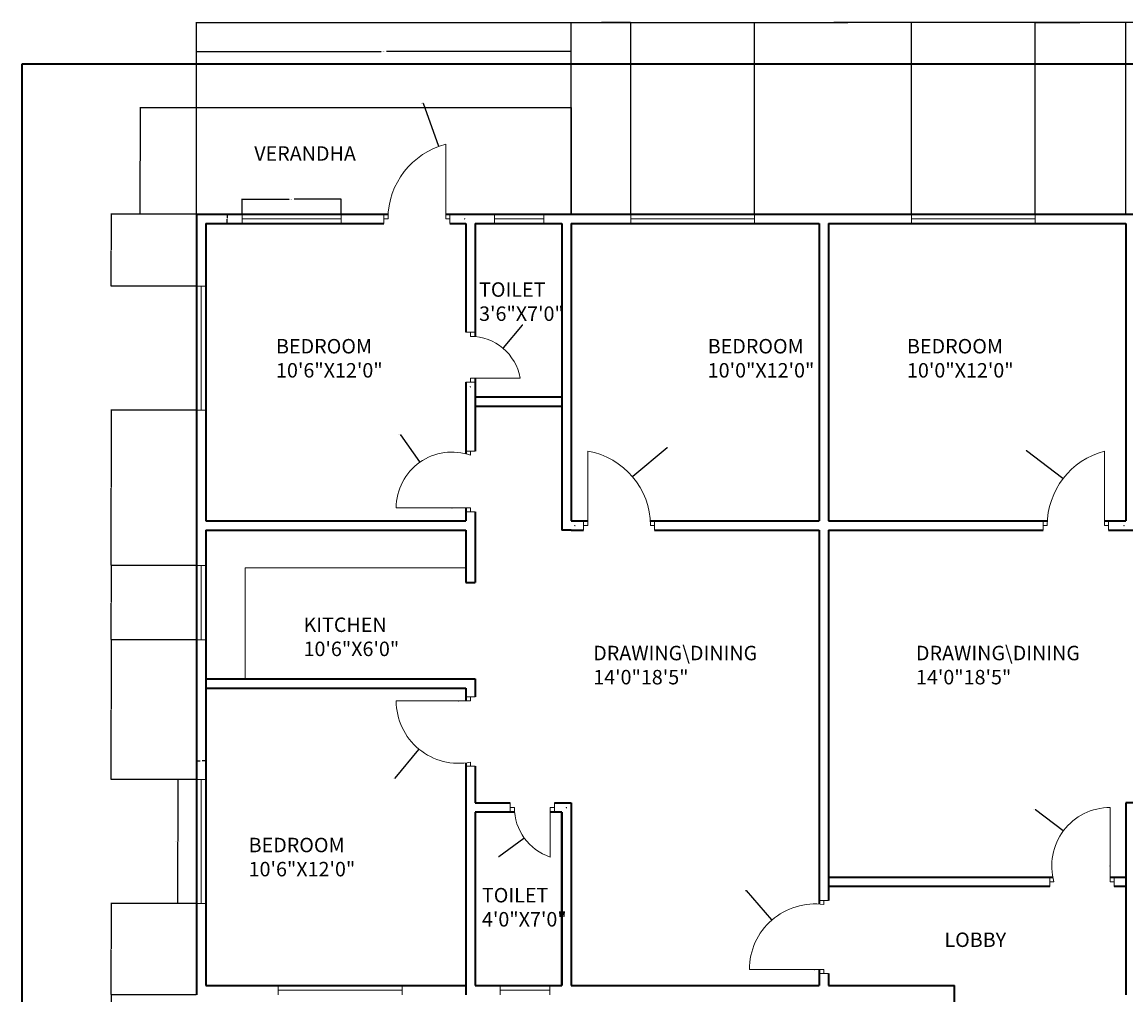
# Model space of a CAD drawing. Units: inches. Extents: x 6393 to 7221, y 6416 to 7347.
# Tile 2 of 3: x 6393 to 6927, y 6876 to 7347. Entities that reach past the tile are written whole.
import ezdxf

# ---------------------------------------------------------------- set-up
doc = ezdxf.new("R2010")
doc.units = ezdxf.units.IN
for name, color, linetype, lineweight in [('A-ANNO-DIMS', 2, 'Continuous', 18), ('A-ANNO-TTLB', 7, 'Continuous', 35), ('A-AREA-IDEN', 7, 'Continuous', 18), ('A-DOOR', 3, 'Continuous', 18), ('A-FLOR-BALC', 7, 'Continuous', 25), ('A-FLOR-FIXT', 8, 'Continuous', 18), ('A-GLAZ', 4, 'Continuous', 18), ('A-WALL', 7, 'Continuous', 35)]:
    doc.layers.add(name, color=color, linetype=linetype, lineweight=lineweight)
doc.styles.get("Standard").update_dxf_attribs({"font": 'arial.ttf'})
doc.dimstyles.get("Standard").update_dxf_attribs({"dimtxt": 0.18, "dimasz": 0.18, "dimexe": 0.18, "dimexo": 0.0625, "dimgap": 0.09, "dimtad": 0, "dimtih": 1, "dimtoh": 1, "dimdec": 4, "dimzin": 0, "dimdsep": 46, "dimtxsty": 'Standard', "dimcen": 0.09, "dimadec": 0, "dimazin": 0, "dimtfac": 1, "dimtdec": 4, "dimtofl": 0, "dimtmove": 0, "dimatfit": 3, "dimfxl": 1, "dimtolj": 1, "dimtzin": 0, "dimarcsym": 0})

# ---------------------------------------------------------------- blocks, each defined once
blk = doc.blocks.new('WIN-60IN')
for p, q in [((0, 60), (4.5, 60)), ((4.5, 60), (2.25, 60)), ((2.25, 60), (2.25, 0)), ((2.25, 0), (0, 0)), ((0, 0), (4.5, 0))]:
    blk.add_line(p, q)
blk = doc.blocks.new('WIN-24IN')
for p, q in [((0, 4.5), (0, 0)), ((0, 0), (0, 2.25)), ((0, 2.25), (24, 2.25)), ((24, 2.25), (24, 4.5)), ((24, 4.5), (24, 0))]:
    blk.add_line(p, q)
blk = doc.blocks.new('WIN-48IN')
for p, q in [((0, 4.5), (0, 0)), ((0, 0), (0, 2.25)), ((0, 2.25), (48, 2.25)), ((48, 2.25), (48, 4.5)), ((48, 4.5), (48, 0))]:
    blk.add_line(p, q)
blk = doc.blocks.new('VERANDA-EDGE')
for p, q in [((0, 0), (0, 51.5)), ((0, 51.5), (181.5, 51.5)), ((181.5, 51.5), (181.5, 0))]:
    blk.add_line(p, q)
blk = doc.blocks.new('*D5')
at = {"layer": 'A-ANNO-DIMS', "color": 0, "lineweight": -2, "transparency": 16777216}
for p, q in [((6476.86, 6980.61), (6467.75, 6980.61)), ((6467.93, 6980.43), (6467.93, 6950.79)), ((6467.93, 6920.79), (6467.93, 6950.43)), ((6476.86, 6920.61), (6467.75, 6920.61))]:
    blk.add_line(p, q, dxfattribs=at)
at = {"layer": 'A-ANNO-DIMS', "color": 0, "transparency": 16777216}
for points in [[(6467.9, 6980.43), (6467.96, 6980.43), (6467.93, 6980.61)], [(6467.9, 6920.79), (6467.96, 6920.79), (6467.93, 6920.61)]]:
    blk.add_solid(points, dxfattribs=at)
at = {"layer": 'Defpoints', "color": 0, "transparency": 16777216}
for p in [(6476.93, 6980.61), (6467.93, 6920.61), (6476.93, 6920.61)]:
    blk.add_point(p, dxfattribs=at)
at = {"layer": 'A-ANNO-DIMS', "color": 0, "transparency": 16777216, "insert": (6467.93, 6950.61), "char_height": 0.18, "attachment_point": 5}
blk.add_mtext('\\A1;WINDOW A 60 TYP.', dxfattribs=at)
blk = doc.blocks.new('*D6')
at = {"layer": 'A-ANNO-DIMS', "color": 0, "lineweight": -2, "transparency": 16777216}
for p, q in [((6476.93, 6980.67), (6476.93, 6989.79)), ((6477.11, 6989.61), (6478.72, 6989.61)), ((6481.25, 6989.61), (6479.64, 6989.61)), ((6481.43, 6980.67), (6481.43, 6989.79))]:
    blk.add_line(p, q, dxfattribs=at)
at = {"layer": 'A-ANNO-DIMS', "color": 0, "transparency": 16777216}
for points in [[(6477.11, 6989.64), (6477.11, 6989.58), (6476.93, 6989.61)], [(6481.25, 6989.64), (6481.25, 6989.58), (6481.43, 6989.61)]]:
    blk.add_solid(points, dxfattribs=at)
at = {"layer": 'Defpoints', "color": 0, "transparency": 16777216}
for p in [(6476.93, 6989.61), (6476.93, 6980.61), (6481.43, 6980.61)]:
    blk.add_point(p, dxfattribs=at)
at = {"layer": 'A-ANNO-DIMS', "color": 0, "transparency": 16777216, "insert": (6479.18, 6989.61), "char_height": 0.18, "attachment_point": 5}
blk.add_mtext('\\A1;5 TYP.', dxfattribs=at)
blk = doc.blocks.new('*D9')
at = {"layer": 'A-ANNO-DIMS', "color": 0, "lineweight": -2, "transparency": 16777216}
for p, q in [((6499.09, 7254.39), (6499.09, 7261.71)), ((6499.27, 7261.53), (6521.85, 7261.53)), ((6546.91, 7261.53), (6524.34, 7261.53)), ((6547.09, 7254.39), (6547.09, 7261.71))]:
    blk.add_line(p, q, dxfattribs=at)
at = {"layer": 'A-ANNO-DIMS', "color": 0, "transparency": 16777216}
for points in [[(6499.27, 7261.56), (6499.27, 7261.5), (6499.09, 7261.53)], [(6546.91, 7261.56), (6546.91, 7261.5), (6547.09, 7261.53)]]:
    blk.add_solid(points, dxfattribs=at)
at = {"layer": 'Defpoints', "color": 0, "transparency": 16777216}
for p in [(6547.09, 7261.53), (6499.09, 7254.33), (6547.09, 7254.33)]:
    blk.add_point(p, dxfattribs=at)
at = {"layer": 'A-ANNO-DIMS', "color": 0, "transparency": 16777216, "insert": (6523.09, 7261.53), "char_height": 0.18, "attachment_point": 5}
blk.add_mtext('\\A1;WINDOW C 48 TYP.', dxfattribs=at)
blk = doc.blocks.new('*D10')
at = {"layer": 'A-ANNO-DIMS', "color": 0, "lineweight": -2, "transparency": 16777216}
for p, q in [((6499.03, 7254.33), (6491.71, 7254.33)), ((6491.89, 7254.15), (6491.89, 7252.26)), ((6499.03, 7249.83), (6491.71, 7249.83)), ((6491.89, 7250.01), (6491.89, 7251.9))]:
    blk.add_line(p, q, dxfattribs=at)
at = {"layer": 'A-ANNO-DIMS', "color": 0, "transparency": 16777216}
for points in [[(6491.86, 7254.15), (6491.92, 7254.15), (6491.89, 7254.33)], [(6491.86, 7250.01), (6491.92, 7250.01), (6491.89, 7249.83)]]:
    blk.add_solid(points, dxfattribs=at)
at = {"layer": 'Defpoints', "color": 0, "transparency": 16777216}
for p in [(6491.89, 7254.33), (6499.09, 7254.33), (6499.09, 7249.83)]:
    blk.add_point(p, dxfattribs=at)
at = {"layer": 'A-ANNO-DIMS', "color": 0, "transparency": 16777216, "insert": (6491.89, 7252.08), "char_height": 0.18, "attachment_point": 5}
blk.add_mtext('\\A1;5 TYP.', dxfattribs=at)
blk = doc.blocks.new('*D11')
at = {"layer": 'A-ANNO-DIMS', "color": 0, "lineweight": -2, "transparency": 16777216}
for p, q in [((6476.93, 7305.89), (6476.93, 7333.23)), ((6477.11, 7333.05), (6566.43, 7333.05)), ((6658.25, 7333.05), (6568.92, 7333.05)), ((6658.43, 7305.89), (6658.43, 7333.23))]:
    blk.add_line(p, q, dxfattribs=at)
at = {"layer": 'A-ANNO-DIMS', "color": 0, "transparency": 16777216}
for points in [[(6477.11, 7333.08), (6477.11, 7333.02), (6476.93, 7333.05)], [(6658.25, 7333.08), (6658.25, 7333.02), (6658.43, 7333.05)]]:
    blk.add_solid(points, dxfattribs=at)
at = {"layer": 'Defpoints', "color": 0, "transparency": 16777216}
for p in [(6658.43, 7333.05), (6476.93, 7305.82), (6658.43, 7305.82)]:
    blk.add_point(p, dxfattribs=at)
at = {"layer": 'A-ANNO-DIMS', "color": 0, "transparency": 16777216, "insert": (6567.68, 7333.05), "char_height": 0.18, "attachment_point": 5}
blk.add_mtext('\\A1;VERANDA 182 TYP.', dxfattribs=at)
blk = doc.blocks.new('*D12')
at = {"layer": 'A-ANNO-DIMS', "color": 0, "lineweight": -2, "transparency": 16777216}
for p, q in [((6476.86, 7305.82), (6449.52, 7305.82)), ((6449.7, 7305.64), (6449.7, 7280.26)), ((6449.7, 7254.51), (6449.7, 7279.89)), ((6476.86, 7254.33), (6449.52, 7254.33))]:
    blk.add_line(p, q, dxfattribs=at)
at = {"layer": 'A-ANNO-DIMS', "color": 0, "transparency": 16777216}
for points in [[(6449.67, 7305.64), (6449.73, 7305.64), (6449.7, 7305.82)], [(6449.67, 7254.51), (6449.73, 7254.51), (6449.7, 7254.33)]]:
    blk.add_solid(points, dxfattribs=at)
at = {"layer": 'Defpoints', "color": 0, "transparency": 16777216}
for p in [(6449.7, 7305.82), (6476.93, 7305.82), (6476.93, 7254.33)]:
    blk.add_point(p, dxfattribs=at)
at = {"layer": 'A-ANNO-DIMS', "color": 0, "transparency": 16777216, "insert": (6449.7, 7280.07), "char_height": 0.18, "attachment_point": 5}
blk.add_mtext('\\A1;51 TYP.', dxfattribs=at)
blk = doc.blocks.new('*D13')
at = {"layer": 'A-ANNO-DIMS', "color": 0, "lineweight": -2, "transparency": 16777216}
for p, q in [((6476.93, 7305.89), (6476.93, 7347.25)), ((6477.11, 7347.07), (6792.33, 7347.07)), ((7108.35, 7347.07), (6793.12, 7347.07)), ((7108.53, 7305.89), (7108.53, 7347.25))]:
    blk.add_line(p, q, dxfattribs=at)
at = {"layer": 'A-ANNO-DIMS', "color": 0, "transparency": 16777216}
for points in [[(6477.11, 7347.1), (6477.11, 7347.04), (6476.93, 7347.07)], [(7108.35, 7347.1), (7108.35, 7347.04), (7108.53, 7347.07)]]:
    blk.add_solid(points, dxfattribs=at)
at = {"layer": 'Defpoints', "color": 0, "transparency": 16777216}
for p in [(7108.53, 7347.07), (6476.93, 7305.82), (7108.53, 7305.82)]:
    blk.add_point(p, dxfattribs=at)
at = {"layer": 'A-ANNO-DIMS', "color": 0, "transparency": 16777216, "insert": (6792.73, 7347.07), "char_height": 0.18, "attachment_point": 5}
blk.add_mtext('\\A1;631.6', dxfattribs=at)
blk = doc.blocks.new('*D16')
at = {"layer": 'A-ANNO-DIMS', "color": 0, "lineweight": -2, "transparency": 16777216}
for p, q in [((6476.86, 6876.33), (6435.5, 6876.33)), ((6435.68, 6876.15), (6435.68, 6864.51)), ((6435.68, 6852.51), (6435.68, 6864.15)), ((6476.86, 6852.33), (6435.5, 6852.33))]:
    blk.add_line(p, q, dxfattribs=at)
at = {"layer": 'A-ANNO-DIMS', "color": 0, "transparency": 16777216}
for points in [[(6435.65, 6876.15), (6435.71, 6876.15), (6435.68, 6876.33)], [(6435.65, 6852.51), (6435.71, 6852.51), (6435.68, 6852.33)]]:
    blk.add_solid(points, dxfattribs=at)
at = {"layer": 'Defpoints', "color": 0, "transparency": 16777216}
for p in [(6435.68, 6876.33), (6476.93, 6876.33), (6476.93, 6852.33)]:
    blk.add_point(p, dxfattribs=at)
at = {"layer": 'A-ANNO-DIMS', "color": 0, "transparency": 16777216, "insert": (6435.68, 6864.33), "char_height": 0.18, "attachment_point": 5}
blk.add_mtext('\\A1;24', dxfattribs=at)
blk = doc.blocks.new('*D17')
at = {"layer": 'A-ANNO-DIMS', "color": 0, "lineweight": -2, "transparency": 16777216}
for p, q in [((6476.86, 6920.61), (6435.5, 6920.61)), ((6435.68, 6920.43), (6435.68, 6898.65)), ((6435.68, 6876.51), (6435.68, 6898.29)), ((6476.86, 6876.33), (6435.5, 6876.33))]:
    blk.add_line(p, q, dxfattribs=at)
at = {"layer": 'A-ANNO-DIMS', "color": 0, "transparency": 16777216}
for points in [[(6435.65, 6920.43), (6435.71, 6920.43), (6435.68, 6920.61)], [(6435.65, 6876.51), (6435.71, 6876.51), (6435.68, 6876.33)]]:
    blk.add_solid(points, dxfattribs=at)
at = {"layer": 'Defpoints', "color": 0, "transparency": 16777216}
for p in [(6435.68, 6920.61), (6476.93, 6920.61), (6476.93, 6876.33)]:
    blk.add_point(p, dxfattribs=at)
at = {"layer": 'A-ANNO-DIMS', "color": 0, "transparency": 16777216, "insert": (6435.68, 6898.47), "char_height": 0.18, "attachment_point": 5}
blk.add_mtext('\\A1;44.285', dxfattribs=at)
blk = doc.blocks.new('*D18')
at = {"layer": 'A-ANNO-DIMS', "color": 0, "lineweight": -2, "transparency": 16777216}
for p, q in [((6476.86, 7048.16), (6435.5, 7048.16)), ((6435.68, 7047.98), (6435.68, 7014.57)), ((6435.68, 6980.79), (6435.68, 7014.2)), ((6476.86, 6980.61), (6435.5, 6980.61))]:
    blk.add_line(p, q, dxfattribs=at)
at = {"layer": 'A-ANNO-DIMS', "color": 0, "transparency": 16777216}
for points in [[(6435.65, 7047.98), (6435.71, 7047.98), (6435.68, 7048.16)], [(6435.65, 6980.79), (6435.71, 6980.79), (6435.68, 6980.61)]]:
    blk.add_solid(points, dxfattribs=at)
at = {"layer": 'Defpoints', "color": 0, "transparency": 16777216}
for p in [(6435.68, 7048.16), (6476.93, 7048.16), (6476.93, 6980.61)]:
    blk.add_point(p, dxfattribs=at)
at = {"layer": 'A-ANNO-DIMS', "color": 0, "transparency": 16777216, "insert": (6435.68, 7014.38), "char_height": 0.18, "attachment_point": 5}
blk.add_mtext('\\A1;67.55', dxfattribs=at)
blk = doc.blocks.new('*D19')
at = {"layer": 'A-ANNO-DIMS', "color": 0, "lineweight": -2, "transparency": 16777216}
for p, q in [((6476.86, 7084.16), (6435.5, 7084.16)), ((6435.68, 7083.98), (6435.68, 7066.34)), ((6435.68, 7048.34), (6435.68, 7065.98)), ((6476.86, 7048.16), (6435.5, 7048.16))]:
    blk.add_line(p, q, dxfattribs=at)
at = {"layer": 'A-ANNO-DIMS', "color": 0, "transparency": 16777216}
for points in [[(6435.65, 7083.98), (6435.71, 7083.98), (6435.68, 7084.16)], [(6435.65, 7048.34), (6435.71, 7048.34), (6435.68, 7048.16)]]:
    blk.add_solid(points, dxfattribs=at)
at = {"layer": 'Defpoints', "color": 0, "transparency": 16777216}
for p in [(6435.68, 7084.16), (6476.93, 7084.16), (6476.93, 7048.16)]:
    blk.add_point(p, dxfattribs=at)
at = {"layer": 'A-ANNO-DIMS', "color": 0, "transparency": 16777216, "insert": (6435.68, 7066.16), "char_height": 0.18, "attachment_point": 5}
blk.add_mtext('\\A1;36', dxfattribs=at)
blk = doc.blocks.new('*D20')
at = {"layer": 'A-ANNO-DIMS', "color": 0, "lineweight": -2, "transparency": 16777216}
for p, q in [((6476.86, 7159.34), (6435.5, 7159.34)), ((6435.68, 7159.16), (6435.68, 7121.93)), ((6435.68, 7084.34), (6435.68, 7121.57)), ((6476.86, 7084.16), (6435.5, 7084.16))]:
    blk.add_line(p, q, dxfattribs=at)
at = {"layer": 'A-ANNO-DIMS', "color": 0, "transparency": 16777216}
for points in [[(6435.65, 7159.16), (6435.71, 7159.16), (6435.68, 7159.34)], [(6435.65, 7084.34), (6435.71, 7084.34), (6435.68, 7084.16)]]:
    blk.add_solid(points, dxfattribs=at)
at = {"layer": 'Defpoints', "color": 0, "transparency": 16777216}
for p in [(6435.68, 7159.34), (6476.93, 7159.34), (6476.93, 7084.16)]:
    blk.add_point(p, dxfattribs=at)
at = {"layer": 'A-ANNO-DIMS', "color": 0, "transparency": 16777216, "insert": (6435.68, 7121.75), "char_height": 0.18, "attachment_point": 5}
blk.add_mtext('\\A1;75.18', dxfattribs=at)
blk = doc.blocks.new('*D21')
at = {"layer": 'A-ANNO-DIMS', "color": 0, "lineweight": -2, "transparency": 16777216}
for p, q in [((6476.86, 7254.33), (6435.5, 7254.33)), ((6435.68, 7254.15), (6435.68, 7237.01)), ((6435.68, 7219.52), (6435.68, 7236.65)), ((6476.86, 7219.34), (6435.5, 7219.34))]:
    blk.add_line(p, q, dxfattribs=at)
at = {"layer": 'A-ANNO-DIMS', "color": 0, "transparency": 16777216}
for points in [[(6435.65, 7254.15), (6435.71, 7254.15), (6435.68, 7254.33)], [(6435.65, 7219.52), (6435.71, 7219.52), (6435.68, 7219.34)]]:
    blk.add_solid(points, dxfattribs=at)
at = {"layer": 'Defpoints', "color": 0, "transparency": 16777216}
for p in [(6435.68, 7254.33), (6476.93, 7254.33), (6476.93, 7219.34)]:
    blk.add_point(p, dxfattribs=at)
at = {"layer": 'A-ANNO-DIMS', "color": 0, "transparency": 16777216, "insert": (6435.68, 7236.83), "char_height": 0.18, "attachment_point": 5}
blk.add_mtext('\\A1;34.99', dxfattribs=at)
blk = doc.blocks.new('*D26')
at = {"layer": 'A-ANNO-DIMS', "color": 0, "lineweight": -2, "transparency": 16777216}
for p, q in [((6658.43, 7254.39), (6658.43, 7347.25)), ((6658.61, 7347.07), (6672.5, 7347.07)), ((6687.05, 7347.07), (6673.15, 7347.07)), ((6687.23, 7254.39), (6687.23, 7347.25))]:
    blk.add_line(p, q, dxfattribs=at)
at = {"layer": 'A-ANNO-DIMS', "color": 0, "transparency": 16777216}
for points in [[(6658.61, 7347.1), (6658.61, 7347.04), (6658.43, 7347.07)], [(6687.05, 7347.1), (6687.05, 7347.04), (6687.23, 7347.07)]]:
    blk.add_solid(points, dxfattribs=at)
at = {"layer": 'Defpoints', "color": 0, "transparency": 16777216}
for p in [(6687.23, 7347.07), (6658.43, 7254.33), (6687.23, 7254.33)]:
    blk.add_point(p, dxfattribs=at)
at = {"layer": 'A-ANNO-DIMS', "color": 0, "transparency": 16777216, "insert": (6672.83, 7347.07), "char_height": 0.18, "attachment_point": 5}
blk.add_mtext('\\A1;28.8', dxfattribs=at)
blk = doc.blocks.new('*D27')
at = {"layer": 'A-ANNO-DIMS', "color": 0, "lineweight": -2, "transparency": 16777216}
for p, q in [((6747.23, 7254.39), (6747.23, 7347.25)), ((6747.41, 7347.07), (6784.8, 7347.07)), ((6822.98, 7347.07), (6785.58, 7347.07)), ((6823.16, 7254.39), (6823.16, 7347.25))]:
    blk.add_line(p, q, dxfattribs=at)
at = {"layer": 'A-ANNO-DIMS', "color": 0, "transparency": 16777216}
for points in [[(6747.41, 7347.1), (6747.41, 7347.04), (6747.23, 7347.07)], [(6822.98, 7347.1), (6822.98, 7347.04), (6823.16, 7347.07)]]:
    blk.add_solid(points, dxfattribs=at)
at = {"layer": 'Defpoints', "color": 0, "transparency": 16777216}
for p in [(6823.16, 7347.07), (6747.23, 7254.33), (6823.16, 7254.33)]:
    blk.add_point(p, dxfattribs=at)
at = {"layer": 'A-ANNO-DIMS', "color": 0, "transparency": 16777216, "insert": (6785.19, 7347.07), "char_height": 0.18, "attachment_point": 5}
blk.add_mtext('\\A1;75.93', dxfattribs=at)
blk = doc.blocks.new('*D28')
at = {"layer": 'A-ANNO-DIMS', "color": 0, "lineweight": -2, "transparency": 16777216}
for p, q in [((6883.16, 7254.39), (6883.16, 7347.25)), ((6883.34, 7347.07), (6904.7, 7347.07)), ((6926.85, 7347.07), (6905.49, 7347.07)), ((6927.03, 7254.39), (6927.03, 7347.25))]:
    blk.add_line(p, q, dxfattribs=at)
at = {"layer": 'A-ANNO-DIMS', "color": 0, "transparency": 16777216}
for points in [[(6883.34, 7347.1), (6883.34, 7347.04), (6883.16, 7347.07)], [(6926.85, 7347.1), (6926.85, 7347.04), (6927.03, 7347.07)]]:
    blk.add_solid(points, dxfattribs=at)
at = {"layer": 'Defpoints', "color": 0, "transparency": 16777216}
for p in [(6927.03, 7347.07), (6883.16, 7254.33), (6927.03, 7254.33)]:
    blk.add_point(p, dxfattribs=at)
at = {"layer": 'A-ANNO-DIMS', "color": 0, "transparency": 16777216, "insert": (6905.09, 7347.07), "char_height": 0.18, "attachment_point": 5}
blk.add_mtext('\\A1;43.87', dxfattribs=at)
blk = doc.blocks.new('*D34')
at = {"layer": 'A-ANNO-DIMS', "color": 0, "lineweight": -2, "transparency": 16777216}
for p, q in [((6878.78, 7139.94), (6878.96, 7139.94)), ((6878.96, 7139.94), (6896.5, 7126.42)), ((6926.03, 7103.58), (6926.21, 7103.58)), ((6926.12, 7103.49), (6926.12, 7103.67))]:
    blk.add_line(p, q, dxfattribs=at)
at = {"layer": 'A-ANNO-DIMS', "color": 0, "transparency": 16777216}
blk.add_solid([(6896.52, 7126.44), (6896.49, 7126.39), (6896.65, 7126.31)], dxfattribs=at)
at = {"layer": 'Defpoints', "color": 0, "transparency": 16777216}
for p in [(6896.65, 7126.31), (6926.12, 7103.58)]:
    blk.add_point(p, dxfattribs=at)
at = {"layer": 'A-ANNO-DIMS', "color": 0, "transparency": 16777216, "insert": (6878.3, 7139.94), "char_height": 0.18, "attachment_point": 5}
blk.add_mtext('\\A1;R37.22', dxfattribs=at)
blk = doc.blocks.new('*D35')
at = {"layer": 'A-ANNO-DIMS', "color": 0, "lineweight": -2, "transparency": 16777216}
for p, q in [((6586.51, 7307.98), (6586.69, 7307.98)), ((6586.69, 7307.98), (6594.19, 7287.19)), ((6606.76, 7252.08), (6606.94, 7252.08)), ((6606.85, 7251.99), (6606.85, 7252.17))]:
    blk.add_line(p, q, dxfattribs=at)
at = {"layer": 'A-ANNO-DIMS', "color": 0, "transparency": 16777216}
blk.add_solid([(6594.21, 7287.2), (6594.16, 7287.18), (6594.25, 7287.02)], dxfattribs=at)
at = {"layer": 'Defpoints', "color": 0, "transparency": 16777216}
for p in [(6594.25, 7287.02), (6606.85, 7252.08)]:
    blk.add_point(p, dxfattribs=at)
at = {"layer": 'A-ANNO-DIMS', "color": 0, "transparency": 16777216, "insert": (6585.96, 7307.98), "char_height": 0.18, "attachment_point": 5}
blk.add_mtext('\\A1;R37.145', dxfattribs=at)
blk = doc.blocks.new('*D36')
at = {"layer": 'A-ANNO-DIMS', "color": 0, "lineweight": -2, "transparency": 16777216}
for p, q in [((6704.93, 7141.22), (6688.3, 7127.22)), ((6705.11, 7141.22), (6704.93, 7141.22)), ((6660.12, 7103.58), (6660.3, 7103.58)), ((6660.21, 7103.49), (6660.21, 7103.67))]:
    blk.add_line(p, q, dxfattribs=at)
at = {"layer": 'A-ANNO-DIMS', "color": 0, "transparency": 16777216}
blk.add_solid([(6688.28, 7127.24), (6688.32, 7127.2), (6688.16, 7127.11)], dxfattribs=at)
at = {"layer": 'Defpoints', "color": 0, "transparency": 16777216}
for p in [(6688.16, 7127.11), (6660.21, 7103.58)]:
    blk.add_point(p, dxfattribs=at)
at = {"layer": 'A-ANNO-DIMS', "color": 0, "transparency": 16777216, "insert": (6705.66, 7141.22), "char_height": 0.18, "attachment_point": 5}
blk.add_mtext('\\A1;R36.535', dxfattribs=at)
blk = doc.blocks.new('*D39')
at = {"layer": 'A-ANNO-DIMS', "color": 0, "lineweight": -2, "transparency": 16777216}
for p, q in [((6742.88, 6926.88), (6743.06, 6926.88)), ((6743.06, 6926.88), (6755.42, 6912.69)), ((6776.26, 6888.68), (6776.44, 6888.68)), ((6776.35, 6888.59), (6776.35, 6888.77))]:
    blk.add_line(p, q, dxfattribs=at)
at = {"layer": 'A-ANNO-DIMS', "color": 0, "transparency": 16777216}
blk.add_solid([(6755.44, 6912.71), (6755.4, 6912.67), (6755.54, 6912.56)], dxfattribs=at)
at = {"layer": 'Defpoints', "color": 0, "transparency": 16777216}
for p in [(6755.54, 6912.56), (6776.35, 6888.68)]:
    blk.add_point(p, dxfattribs=at)
at = {"layer": 'A-ANNO-DIMS', "color": 0, "transparency": 16777216, "insert": (6742.4, 6926.88), "char_height": 0.18, "attachment_point": 5}
blk.add_mtext('\\A1;R31.67', dxfattribs=at)
blk = doc.blocks.new('*D42')
at = {"layer": 'A-ANNO-DIMS', "color": 0, "lineweight": -2, "transparency": 16777216}
for p, q in [((6603.8, 7018.63), (6603.98, 7018.63)), ((6603.89, 7018.54), (6603.89, 7018.72)), ((6573.16, 6981.32), (6584.57, 6995.18)), ((6572.98, 6981.32), (6573.16, 6981.32))]:
    blk.add_line(p, q, dxfattribs=at)
at = {"layer": 'A-ANNO-DIMS', "color": 0, "transparency": 16777216}
blk.add_solid([(6584.54, 6995.2), (6584.59, 6995.16), (6584.68, 6995.32)], dxfattribs=at)
at = {"layer": 'Defpoints', "color": 0, "transparency": 16777216}
for p in [(6603.89, 7018.63), (6584.68, 6995.32)]:
    blk.add_point(p, dxfattribs=at)
at = {"layer": 'A-ANNO-DIMS', "color": 0, "transparency": 16777216, "insert": (6572.52, 6981.32), "char_height": 0.18, "attachment_point": 5}
blk.add_mtext('\\A1;R30.21', dxfattribs=at)
blk = doc.blocks.new('*D46')
at = {"layer": 'A-ANNO-DIMS', "color": 0, "lineweight": -2, "transparency": 16777216}
for p, q in [((6883.1, 6966.08), (6883.28, 6966.08)), ((6883.28, 6966.08), (6896.68, 6955.96)), ((6919.3, 6938.79), (6919.48, 6938.79)), ((6919.39, 6938.7), (6919.39, 6938.88))]:
    blk.add_line(p, q, dxfattribs=at)
at = {"layer": 'A-ANNO-DIMS', "color": 0, "transparency": 16777216}
blk.add_solid([(6896.7, 6955.98), (6896.66, 6955.93), (6896.82, 6955.85)], dxfattribs=at)
at = {"layer": 'Defpoints', "color": 0, "transparency": 16777216}
for p in [(6896.82, 6955.85), (6919.39, 6938.79)]:
    blk.add_point(p, dxfattribs=at)
at = {"layer": 'A-ANNO-DIMS', "color": 0, "transparency": 16777216, "insert": (6882.62, 6966.08), "char_height": 0.18, "attachment_point": 5}
blk.add_mtext('\\A1;R28.29', dxfattribs=at)
blk = doc.blocks.new('*D47')
at = {"layer": 'A-ANNO-DIMS', "color": 0, "lineweight": -2, "transparency": 16777216}
for p, q in [((6575.6, 7147.39), (6575.78, 7147.39)), ((6575.78, 7147.39), (6584.99, 7134.32)), ((6600.54, 7112.15), (6600.72, 7112.15)), ((6600.63, 7112.06), (6600.63, 7112.24))]:
    blk.add_line(p, q, dxfattribs=at)
at = {"layer": 'A-ANNO-DIMS', "color": 0, "transparency": 16777216}
blk.add_solid([(6585.02, 7134.34), (6584.97, 7134.31), (6585.1, 7134.18)], dxfattribs=at)
at = {"layer": 'Defpoints', "color": 0, "transparency": 16777216}
for p in [(6585.1, 7134.18), (6600.63, 7112.15)]:
    blk.add_point(p, dxfattribs=at)
at = {"layer": 'A-ANNO-DIMS', "color": 0, "transparency": 16777216, "insert": (6575.12, 7147.39), "char_height": 0.18, "attachment_point": 5}
blk.add_mtext('\\A1;R26.95', dxfattribs=at)
blk = doc.blocks.new('*D49')
at = {"layer": 'A-ANNO-DIMS', "color": 0, "lineweight": -2, "transparency": 16777216}
for p, q in [((6656.05, 6967.08), (6656.23, 6967.08)), ((6656.14, 6966.99), (6656.14, 6967.17)), ((6623.43, 6943.36), (6635.55, 6952.15)), ((6623.25, 6943.36), (6623.43, 6943.36))]:
    blk.add_line(p, q, dxfattribs=at)
at = {"layer": 'A-ANNO-DIMS', "color": 0, "transparency": 16777216}
blk.add_solid([(6635.53, 6952.17), (6635.56, 6952.13), (6635.69, 6952.26)], dxfattribs=at)
at = {"layer": 'Defpoints', "color": 0, "transparency": 16777216}
for p in [(6656.14, 6967.08), (6635.69, 6952.26)]:
    blk.add_point(p, dxfattribs=at)
at = {"layer": 'A-ANNO-DIMS', "color": 0, "transparency": 16777216, "insert": (6622.76, 6943.36), "char_height": 0.18, "attachment_point": 5}
blk.add_mtext('\\A1;R25.25', dxfattribs=at)
blk = doc.blocks.new('*D51')
at = {"layer": 'A-ANNO-DIMS', "color": 0, "lineweight": -2, "transparency": 16777216}
for p, q in [((6634.73, 7200.59), (6625.45, 7189.52)), ((6634.91, 7200.59), (6634.73, 7200.59)), ((6609.59, 7170.71), (6609.77, 7170.71)), ((6609.68, 7170.62), (6609.68, 7170.8))]:
    blk.add_line(p, q, dxfattribs=at)
at = {"layer": 'A-ANNO-DIMS', "color": 0, "transparency": 16777216}
blk.add_solid([(6625.43, 7189.54), (6625.48, 7189.5), (6625.34, 7189.38)], dxfattribs=at)
at = {"layer": 'Defpoints', "color": 0, "transparency": 16777216}
for p in [(6625.34, 7189.38), (6609.68, 7170.71)]:
    blk.add_point(p, dxfattribs=at)
at = {"layer": 'A-ANNO-DIMS', "color": 0, "transparency": 16777216, "insert": (6635.46, 7200.59), "char_height": 0.18, "attachment_point": 5}
blk.add_mtext('\\A1;R24.373', dxfattribs=at)

msp = doc.modelspace()

# ---------------------------------------------------------------- linework, layer by layer
at = {"layer": 'A-ANNO-TTLB'}
msp.add_lwpolyline([(6392.5039, 7327.0003), (7221.4173, 7327.0003), (7221.4173, 6416.0496), (6392.5039, 6416.0496)], close=True, dxfattribs=at)
at = {"layer": 'A-DOOR'}
for p, q in [((6597.6967, 7252.0767), (6597.6967, 7288.0767)), ((6567.7037, 7254.3267), (6567.7037, 7249.8267)), ((6599.6967, 7254.3267), (6599.6967, 7249.8267)), ((6567.7037, 7249.8267), (6567.7037, 7252.0767)), ((6567.7037, 7252.0767), (6569.7037, 7252.0767)), ((6599.6967, 7252.0767), (6597.6967, 7252.0767)), ((6599.6967, 7249.8267), (6599.6967, 7252.0767)), ((6607.4273, 7197.0782), (6611.9273, 7197.0782)), ((6611.9273, 7197.0782), (6609.6773, 7197.0782)), ((6609.6773, 7197.0782), (6609.6773, 7195.0782)), ((6609.6773, 7172.9523), (6609.6773, 7174.9523)), ((6609.6773, 7174.9523), (6633.6773, 7174.9523)), ((6611.9273, 7172.9523), (6607.4273, 7172.9523)), ((6607.4273, 7172.9523), (6609.6773, 7172.9523)), ((6607.4273, 7139.5396), (6611.9273, 7139.5396)), ((6611.9273, 7139.5396), (6609.6773, 7139.5396)), ((6609.6773, 7139.5396), (6609.6773, 7137.5396)), ((6666.439, 7103.5767), (6666.439, 7139.5767)), ((6916.6614, 7103.5767), (6916.6614, 7139.5767)), ((6609.6773, 7112.1517), (6573.6773, 7112.1517)), ((6607.4273, 7110.1517), (6611.9273, 7110.1517)), ((6609.6773, 7110.1517), (6609.6773, 7112.1517)), ((6611.9273, 7110.1517), (6609.6773, 7110.1517)), ((6664.439, 7105.8267), (6664.439, 7101.3267)), ((6698.7463, 7105.8267), (6698.7463, 7101.3267)), ((6886.9016, 7105.8267), (6886.9016, 7101.3267)), ((6918.6614, 7105.8267), (6918.6614, 7101.3267)), ((6664.439, 7101.3267), (6664.439, 7103.5767)), ((6664.439, 7103.5767), (6666.439, 7103.5767)), ((6698.7463, 7103.5767), (6696.7463, 7103.5767)), ((6698.7463, 7101.3267), (6698.7463, 7103.5767)), ((6886.9016, 7101.3267), (6886.9016, 7103.5767)), ((6886.9016, 7103.5767), (6888.9016, 7103.5767)), ((6918.6614, 7103.5767), (6916.6614, 7103.5767)), ((6918.6614, 7101.3267), (6918.6614, 7103.5767)), ((6609.6773, 7018.6341), (6573.6773, 7018.6341)), ((6611.9273, 7020.6341), (6607.4273, 7020.6341)), ((6607.4273, 7020.6341), (6609.6773, 7020.6341)), ((6609.6773, 7020.6341), (6609.6773, 7018.6341)), ((6607.4273, 6986.9854), (6611.9273, 6986.9854)), ((6609.6773, 6986.9854), (6609.6773, 6988.9854)), ((6611.9273, 6986.9854), (6609.6773, 6986.9854)), ((6628.8848, 6969.3267), (6628.8848, 6964.8267)), ((6628.8848, 6964.8267), (6628.8848, 6967.0767)), ((6628.8848, 6967.0767), (6630.8848, 6967.0767)), ((6650.2836, 6967.0767), (6648.2836, 6967.0767)), ((6648.2836, 6967.0767), (6648.2836, 6943.0767)), ((6650.2836, 6969.3267), (6650.2836, 6964.8267)), ((6650.2836, 6964.8267), (6650.2836, 6967.0767)), ((6919.3865, 6931.0767), (6919.3865, 6967.0767)), ((6890.1686, 6933.3267), (6890.1686, 6928.8267)), ((6921.3865, 6933.3267), (6921.3865, 6928.8267)), ((6890.1686, 6928.8267), (6890.1686, 6931.0767)), ((6890.1686, 6931.0767), (6892.1686, 6931.0767)), ((6921.3865, 6931.0767), (6919.3865, 6931.0767)), ((6921.3865, 6928.8267), (6921.3865, 6931.0767)), ((6778.4273, 6922.055), (6782.9273, 6922.055)), ((6782.9273, 6922.055), (6778.4273, 6922.055)), ((6778.4273, 6922.055), (6780.6773, 6922.055)), ((6780.6773, 6922.055), (6780.6773, 6920.055)), ((6780.6773, 6888.6821), (6744.6773, 6888.6821)), ((6778.4273, 6886.6821), (6782.9273, 6886.6821)), ((6780.6773, 6886.6821), (6780.6773, 6888.6821)), ((6782.9273, 6886.6821), (6780.6773, 6886.6821))]:
    msp.add_line(p, q, dxfattribs=at)
for centre, radius, start, end in [((6606.8488, 7252.0767), 37.1451, 104.263921, 180), ((6609.6773, 7170.7053), 24.3729, 10.034948, 90), ((6600.6293, 7112.1517), 26.952, 70.384423, 180), ((6660.2116, 7103.5767), 36.5346, 0, 80.185967), ((6926.1246, 7103.5767), 37.223, 104.727922, 180), ((6603.8862, 7018.6341), 30.2089, 180, 281.052013), ((6656.137, 6967.0767), 25.2523, 180, 251.880499), ((6919.3865, 6938.7877), 28.2891, 90, 195.817656), ((6776.3475, 6888.6821), 31.6702, 82.142259, 180)]:
    msp.add_arc(centre, radius, start, end, dxfattribs=at)
at = {"layer": 'A-FLOR-FIXT'}
for p, q in [((6607.4273, 7083.05), (6500.4821, 7083.05)), ((6500.4821, 7083.05), (6500.4821, 7029.3267))]:
    msp.add_line(p, q, dxfattribs=at)
at = {"layer": 'A-GLAZ'}
for p, q in [((6481.4273, 7084.1574), (6476.9273, 7084.1574)), ((6476.9273, 7084.1574), (6479.1773, 7084.1574)), ((6479.1773, 7084.1574), (6479.1773, 7060.1574)), ((6479.1773, 7060.1574), (6479.1773, 7048.1574)), ((6479.1773, 7048.1574), (6476.9273, 7048.1574)), ((6476.9273, 7048.1574), (6481.4273, 7048.1574))]:
    msp.add_line(p, q, dxfattribs=at)
at = {"layer": 'A-WALL'}
for p, q in [((6476.9273, 7254.3267), (6476.9273, 6876.3267)), ((6476.9273, 7254.3267), (6569.7719, 7254.3267)), ((6476.9273, 7254.3267), (6569.7719, 7254.3267)), ((6597.6967, 7254.3267), (6985.3208, 7254.3267)), ((6597.6967, 7254.3267), (6985.3208, 7254.3267)), ((6481.4273, 7249.8267), (6567.7037, 7249.8267)), ((6481.4273, 7249.8267), (6481.4273, 7105.8267)), ((6599.6967, 7249.8267), (6607.4273, 7249.8267)), ((6607.4273, 7249.8267), (6607.4273, 7197.0782)), ((6611.9273, 7249.8267), (6611.9273, 7194.9741)), ((6611.9273, 7249.8267), (6653.9273, 7249.8267)), ((6653.9273, 7249.8267), (6653.9273, 7101.3267)), ((6658.4273, 7249.8267), (6658.4273, 7105.8267)), ((6658.4273, 7249.8267), (6778.4273, 7249.8267)), ((6778.4273, 7249.8267), (6778.4273, 7105.8267)), ((6782.9273, 7249.8267), (6782.9273, 7105.8267)), ((6782.9273, 7249.8267), (6926.9273, 7249.8267)), ((6926.9273, 7249.8267), (6926.9273, 7105.8267)), ((6611.9273, 7174.9523), (6611.9273, 7139.5396)), ((6607.4273, 7172.9523), (6607.4273, 7138.2323)), ((6611.9273, 7165.8267), (6653.9273, 7165.8267)), ((6611.9273, 7161.3267), (6653.9273, 7161.3267)), ((6607.4273, 7112.1517), (6607.4273, 7105.8267)), ((6611.9273, 7110.1517), (6611.9273, 7075.9844)), ((6481.4273, 7105.8267), (6607.4273, 7105.8267)), ((6658.4273, 7105.8267), (6666.439, 7105.8267)), ((6696.6769, 7105.8267), (6778.4273, 7105.8267)), ((6782.9273, 7105.8267), (6888.9696, 7105.8267)), ((6916.6614, 7105.8267), (6926.9273, 7105.8267)), ((6481.4273, 7101.3267), (6607.4273, 7101.3267)), ((6481.4273, 7101.3267), (6481.4273, 6880.8267)), ((6607.4273, 7101.3267), (6607.4273, 7075.9844)), ((6658.4273, 7101.3267), (6653.9273, 7101.3267)), ((6658.4273, 7101.3267), (6664.439, 7101.3267)), ((6698.7463, 7101.3267), (6778.4273, 7101.3267)), ((6778.4273, 7101.3267), (6778.4273, 6920.284)), ((6782.9273, 7101.3267), (6886.9016, 7101.3267)), ((6782.9273, 7101.3267), (6782.9273, 6922.055)), ((6782.9273, 7101.3267), (6782.9273, 6933.3267)), ((6918.6614, 7101.3267), (6931.4273, 7101.3267)), ((6607.4273, 7075.9844), (6611.9273, 7075.9844)), ((6481.4273, 7029.3267), (6607.4273, 7029.3267)), ((6607.4273, 7029.3267), (6611.9273, 7029.3267)), ((6611.9273, 7029.3267), (6611.9273, 7020.6341)), ((6481.4273, 7024.8267), (6607.4273, 7024.8267)), ((6607.4273, 7024.8267), (6607.4273, 7018.6341)), ((6607.4273, 6988.6334), (6607.4273, 6880.8267)), ((6611.9273, 6986.9854), (6611.9273, 6969.3267)), ((6611.9273, 6969.3267), (6628.8848, 6969.3267)), ((6650.2836, 6969.3267), (6658.4273, 6969.3267)), ((6658.4273, 6969.3267), (6658.4273, 6880.8267)), ((6926.9273, 6969.3267), (6926.9273, 6876.3267)), ((6935.1409, 6969.3267), (6926.9273, 6969.3267)), ((6630.9852, 6964.8267), (6611.9273, 6964.8267)), ((6611.9273, 6964.8267), (6611.9273, 6880.8267)), ((6653.9273, 6964.8267), (6648.2836, 6964.8267)), ((6653.9273, 6880.8267), (6653.9273, 6964.8267)), ((6653.9273, 6964.8267), (6653.9273, 6880.8267)), ((6782.9273, 6933.3267), (6891.6295, 6933.3267)), ((6919.3865, 6933.3267), (6926.9273, 6933.3267)), ((6926.9273, 6933.3267), (6926.9273, 6928.8267)), ((6890.1686, 6928.8267), (6782.9273, 6928.8267)), ((6926.9273, 6928.8267), (6921.3865, 6928.8267)), ((6778.4273, 6888.6821), (6778.4273, 6880.8267)), ((6782.9273, 6886.6821), (6782.9273, 6880.8267)), ((6481.4273, 6880.8267), (6607.4273, 6880.8267)), ((6481.4273, 6880.8267), (6607.4273, 6880.8267)), ((6607.4273, 6880.8267), (6607.4273, 6876.3267)), ((6611.9273, 6880.8267), (6653.9273, 6880.8267)), ((6658.4273, 6880.8267), (6778.4273, 6880.8267)), ((6782.9273, 6880.8267), (6843.9675, 6880.8267)), ((6843.9675, 6852.3267), (6843.9675, 6880.8267))]:
    msp.add_line(p, q, dxfattribs=at)

# ---------------------------------------------------------------- block references
at = {"layer": 'A-FLOR-BALC'}
msp.add_blockref('VERANDA-EDGE', (6476.927, 7254.327), dxfattribs=at)
at = {"layer": 'A-GLAZ'}
for name, p in [('WIN-48IN', (6499.093, 7249.827)), ('WIN-24IN', (6621.218, 7249.827)), ('WIN-60IN', (6476.927, 7159.338)), ('WIN-24IN', (6623.9861, 6876.327))]:
    msp.add_blockref(name, p, dxfattribs=at)
at = {"layer": 'A-GLAZ', "extrusion": (0, 0, -1), "zscale": -1, "rotation": 270}
for p in [(-6747.2253, 7254.327), (-6883.1587, 7254.327), (-6576.5769, 6880.827)]:
    msp.add_blockref('WIN-60IN', p, dxfattribs=at)
at = {"layer": 'A-GLAZ', "rotation": 180}
msp.add_blockref('WIN-60IN', (6481.4275, 6980.6121), dxfattribs=at)

# ---------------------------------------------------------------- texts
at = {"layer": 'A-AREA-IDEN', "char_height": 7, "attachment_point": 1}
for s, width, insert in [('VERANDHA', 116.976107, (6504.9304, 7287.126)), ('TOILET\\P3\'6"X7\'0"', 71.069921, (6613.8066, 7221.2778)), ('BEDROOM\\P10\'6"X12\'0"', 101.475202, (6515.4735, 7193.8445)), ('BEDROOM\\P10\'0"X12\'0"', 101.475202, (6724.5133, 7193.8445)), ('BEDROOM\\P10\'0"X12\'0"', 101.475202, (6821.0125, 7193.8445)), ('KITCHEN\\P10\'6"X6\'0"', 100.143282, (6528.7949, 7059.0096)), ('DRAWING\\\\DINING\\P14\'0"18\'5"', 91.848577, (6669.0667, 7045.318)), ('DRAWING\\\\DINING\\P14\'0"18\'5"', 91.848577, (6825.3593, 7045.318)), ('BEDROOM\\P10\'6"X12\'0"', 113.517557, (6502.2028, 6952.388)), ('TOILET\\P4\'0"X7\'0"', 104.595174, (6615.1829, 6928.1036)), ('LOBBY', 43.743622, (6839.1394, 6906.5282))]:
    msp.add_mtext_dynamic_manual_height_columns(s, width=width, gutter_width=12.5, heights=[0], dxfattribs=dict(at, insert=insert))

# ---------------------------------------------------------------- dimensions: what is measured, and where the dimension line sits
at = {"layer": 'A-ANNO-DIMS'}
for base, p1, p2, override, picture, middle in [((7108.5274, 7347.0726), (6476.9273, 7305.8226), (7108.5274, 7305.8226), {"dimdec": 1, "dimlfac": 1, "dimrnd": 0, "dimzin": 0, "dimdsep": 46, "dimlunit": 2}, '*D13', (6792.7273, 7347.0726)), ((6687.2251, 7347.0726), (6658.4273, 7254.3267), (6687.2251, 7254.3267), {"dimdec": 1, "dimlfac": 1, "dimrnd": 0, "dimzin": 0, "dimdsep": 46, "dimlunit": 2}, '*D26', (6672.8262, 7347.0726)), ((6823.1584, 7347.0726), (6747.2251, 7254.3267), (6823.1584, 7254.3267), {"dimdec": 2, "dimlfac": 1, "dimrnd": 0, "dimzin": 0, "dimdsep": 46, "dimlunit": 2}, '*D27', (6785.1917, 7347.0726)), ((6927.0274, 7347.0726), (6883.1584, 7254.3267), (6927.0274, 7254.3267), {"dimdec": 2, "dimlfac": 1, "dimrnd": 0, "dimzin": 0, "dimdsep": 46, "dimlunit": 2}, '*D28', (6905.0929, 7347.0726))]:
    dim = msp.add_linear_dim(base=base, p1=p1, p2=p2, dimstyle='Standard', override=override, dxfattribs=at)
    dim.commit()
    dim.dimension.update_dxf_attribs({"geometry": picture, "text_midpoint": middle})
for base, p1, p2, text, picture, middle in [((6658.42726952, 7333.047594732), (6476.92726952, 7305.822594732), (6658.42726952, 7305.822594732), 'VERANDA <> TYP.', '*D11', (6567.67726952, 7333.047594732)), ((6547.0925, 7261.5267), (6499.0925, 7254.3267), (6547.0925, 7254.3267), 'WINDOW C <> TYP.', '*D9', (6523.0925, 7261.5267))]:
    dim = msp.add_linear_dim(base=base, p1=p1, p2=p2, text=text, dimstyle='Standard', override={"dimdec": 0, "dimlfac": 1, "dimrnd": 0, "dimzin": 0, "dimdsep": 46, "dimlunit": 2}, dxfattribs=at)
    dim.commit()
    dim.dimension.update_dxf_attribs({"geometry": picture, "text_midpoint": middle})
for center, mpoint, override, picture, middle in [((6606.8488, 7252.0767), (6594.2472, 7287.019), {"dimdec": 3, "dimlfac": 1, "dimrnd": 0, "dimzin": 0, "dimdsep": 46, "dimlunit": 2}, '*D35', (6585.9559, 7307.9844)), ((6609.6773, 7170.7053), (6625.338, 7189.381), {"dimdec": 3, "dimlfac": 1, "dimrnd": 0, "dimzin": 0, "dimdsep": 46, "dimlunit": 2}, '*D51', (6635.4641, 7200.5863)), ((6600.6293, 7112.1517), (6585.0963, 7134.1776), {"dimdec": 2, "dimlfac": 1, "dimrnd": 0, "dimzin": 0, "dimdsep": 46, "dimlunit": 2}, '*D47', (6575.116, 7147.3931)), ((6660.2116, 7103.5767), (6688.1608, 7127.1059), {"dimdec": 3, "dimlfac": 1, "dimrnd": 0, "dimzin": 0, "dimdsep": 46, "dimlunit": 2}, '*D36', (6705.6608, 7141.2234)), ((6926.1246, 7103.5767), (6896.6474, 7126.3067), {"dimdec": 2, "dimlfac": 1, "dimrnd": 0, "dimzin": 0, "dimdsep": 46, "dimlunit": 2}, '*D34', (6878.3022, 7139.9446)), ((6603.8862, 7018.6341), (6584.682, 6995.315), {"dimdec": 2, "dimlfac": 1, "dimrnd": 0, "dimzin": 0, "dimdsep": 46, "dimlunit": 2}, '*D42', (6572.5171, 6981.3236)), ((6656.137, 6967.0767), (6635.6921, 6952.2551), {"dimdec": 2, "dimlfac": 1, "dimrnd": 0, "dimzin": 0, "dimdsep": 46, "dimlunit": 2}, '*D49', (6622.7646, 6943.3621)), ((6919.3865, 6938.7877), (6896.8208, 6955.8481), {"dimdec": 2, "dimlfac": 1, "dimrnd": 0, "dimzin": 0, "dimdsep": 46, "dimlunit": 2}, '*D46', (6882.6214, 6966.0844)), ((6776.3475, 6888.6821), (6755.5401, 6912.5579), {"dimdec": 2, "dimlfac": 1, "dimrnd": 0, "dimzin": 0, "dimdsep": 46, "dimlunit": 2}, '*D39', (6742.3957, 6926.8834))]:
    dim = msp.add_radius_dim(center=center, mpoint=mpoint, dimstyle='Standard', override=override, dxfattribs=at)
    dim.commit()
    dim.dimension.update_dxf_attribs({"geometry": picture, "text_midpoint": middle, "dimtype": 164})
for base, p1, p2, angle, text, picture, middle in [((6449.7023, 7305.8226), (6476.9273, 7254.3267), (6476.9273, 7305.8226), 90, '<> TYP.', '*D12', (6449.7023, 7280.0747)), ((6491.8925291362, 7254.3267298921), (6499.0925291362, 7249.8267298921), (6499.0925291362, 7254.3267298921), 90, '<> TYP.', '*D10', (6491.8925291362, 7252.0767298921)), ((6476.92726952, 6989.6118394049), (6481.42726952, 6980.6118394049), (6476.92726952, 6980.6118394049), 180, '<> TYP.', '*D6', (6479.17726952, 6989.6118394049)), ((6467.9273, 6920.6118), (6476.9273, 6980.6118), (6476.9273, 6920.6118), 270, 'WINDOW A <> TYP.', '*D5', (6467.9273, 6950.6118))]:
    dim = msp.add_linear_dim(base=base, p1=p1, p2=p2, angle=angle, text=text, dimstyle='Standard', override={"dimdec": 0, "dimlfac": 1, "dimrnd": 0, "dimzin": 0, "dimdsep": 46, "dimlunit": 2}, dxfattribs=at)
    dim.commit()
    dim.dimension.update_dxf_attribs({"geometry": picture, "text_midpoint": middle})
for base, p1, p2, override, picture, middle in [((6435.6773, 7254.3267), (6476.9273, 7219.3383), (6476.9273, 7254.3267), {"dimdec": 2, "dimlfac": 1, "dimrnd": 0, "dimzin": 0, "dimdsep": 46, "dimlunit": 2}, '*D21', (6435.6773, 7236.8325)), ((6435.6773, 7159.3383), (6476.9273, 7084.1574), (6476.9273, 7159.3383), {"dimdec": 2, "dimlfac": 1, "dimrnd": 0, "dimzin": 0, "dimdsep": 46, "dimlunit": 2}, '*D20', (6435.6773, 7121.7478)), ((6435.6773, 7084.1574), (6476.9273, 7048.1574), (6476.9273, 7084.1574), {"dimdec": 0, "dimlfac": 1, "dimrnd": 0, "dimzin": 0, "dimdsep": 46, "dimlunit": 2}, '*D19', (6435.6773, 7066.1574)), ((6435.6773, 7048.1574), (6476.9273, 6980.6118), (6476.9273, 7048.1574), {"dimdec": 2, "dimlfac": 1, "dimrnd": 0, "dimzin": 0, "dimdsep": 46, "dimlunit": 2}, '*D18', (6435.6773, 7014.3846)), ((6435.6773, 6920.6118), (6476.9273, 6876.3267), (6476.9273, 6920.6118), {"dimdec": 3, "dimlfac": 1, "dimrnd": 0, "dimzin": 0, "dimdsep": 46, "dimlunit": 2}, '*D17', (6435.6773, 6898.4693)), ((6435.6773, 6876.3267), (6476.9273, 6852.3267), (6476.9273, 6876.3267), {"dimdec": 0, "dimlfac": 1, "dimrnd": 0, "dimzin": 0, "dimdsep": 46, "dimlunit": 2}, '*D16', (6435.6773, 6864.3267))]:
    dim = msp.add_linear_dim(base=base, p1=p1, p2=p2, angle=90, dimstyle='Standard', override=override, dxfattribs=at)
    dim.commit()
    dim.dimension.update_dxf_attribs({"geometry": picture, "text_midpoint": middle})

doc.saveas('drawing.dxf')
